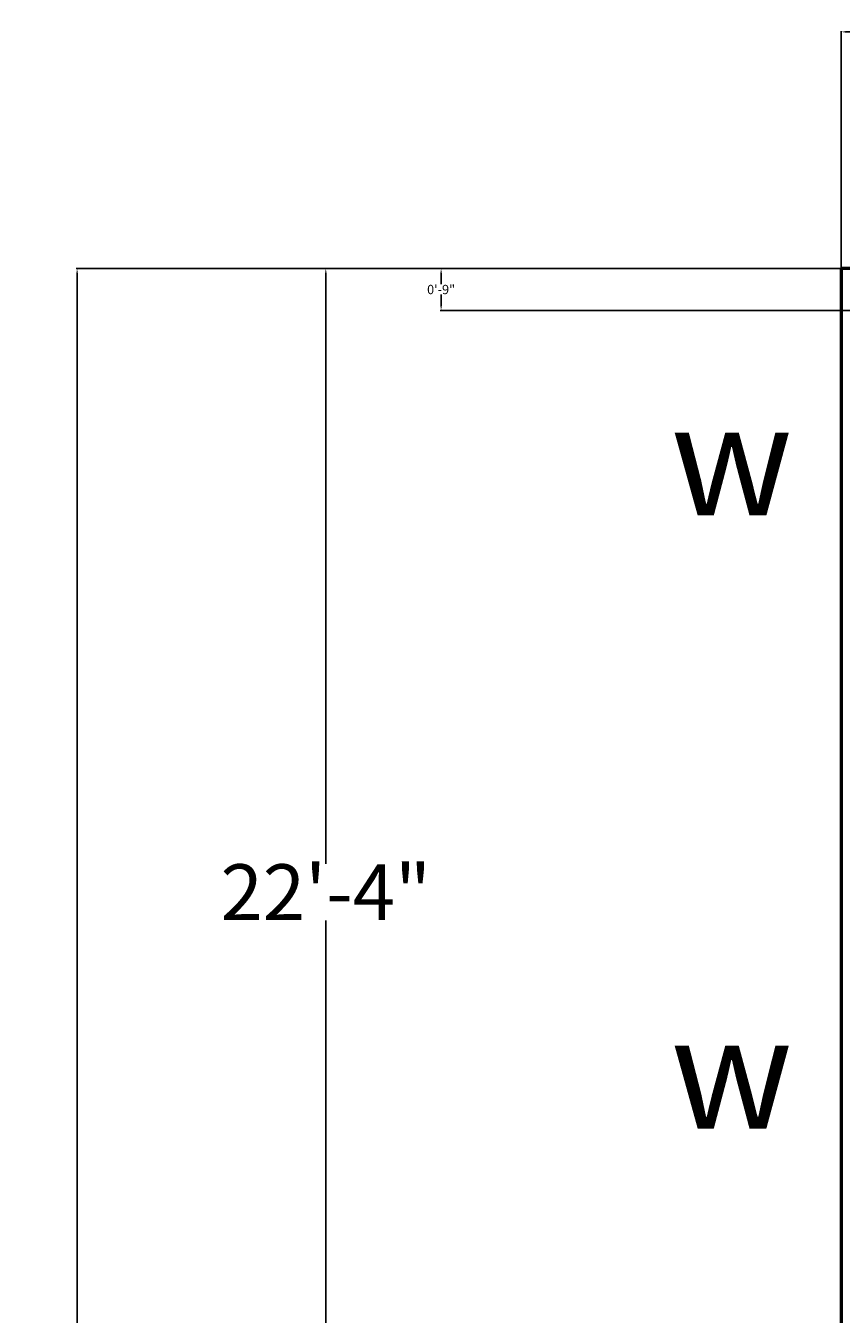
# Model space of a CAD drawing. Units: inches. Extents: x 409 to 7572, y 7 to 725.
# Tile 29 of 38: x 5502 to 5677, y 448 to 725. Entities that reach past the tile are written whole.
import ezdxf

# ---------------------------------------------------------------- set-up
doc = ezdxf.new("R2010")
doc.units = ezdxf.units.IN
doc.header["$MEASUREMENT"] = 0
for name, color, linetype, lineweight in [('A-ANNO-DIMS', 2, 'Continuous', 18), ('A-ANNO-SYMB', 3, 'Continuous', 25), ('A-WALL', 7, 'Continuous', 50)]:
    doc.layers.add(name, color=color, linetype=linetype, lineweight=lineweight)
doc.styles.get("Standard").update_dxf_attribs({"font": 'arial.ttf'})
doc.dimstyles.get("Standard").update_dxf_attribs({"dimtxt": 2, "dimasz": 1, "dimexe": 0.18, "dimexo": 0.0625, "dimgap": 0.09, "dimtad": 0, "dimtih": 1, "dimtoh": 1, "dimdec": 0, "dimzin": 0, "dimdsep": 46, "dimlunit": 3, "dimtxsty": 'Standard', "dimcen": 0.09, "dimadec": 0, "dimazin": 0, "dimtfac": 1, "dimtdec": 0, "dimtofl": 0, "dimtmove": 0, "dimatfit": 3, "dimfxl": 1, "dimtolj": 1, "dimtzin": 0, "dimarcsym": 0})

# ---------------------------------------------------------------- blocks, each defined once
blk = doc.blocks.new('*D146')
at = {"layer": 'A-ANNO-DIMS', "color": 0, "lineweight": -2, "transparency": 16777216}
for p, q in [((5676.78, 672.59), (5676.78, 723.56)), ((5677.78, 723.38), (5944.22, 723.38)), ((6217.78, 723.38), (5951.35, 723.38)), ((6218.78, 672.59), (6218.78, 723.56))]:
    blk.add_line(p, q, dxfattribs=at)
at = {"layer": 'A-ANNO-DIMS', "color": 0, "transparency": 16777216}
for points in [[(5677.78, 723.55), (5677.78, 723.22), (5676.78, 723.38)], [(6217.78, 723.55), (6217.78, 723.22), (6218.78, 723.38)]]:
    blk.add_solid(points, dxfattribs=at)
at = {"layer": 'DEFPOINTS', "color": 0, "transparency": 16777216}
for p in [(5676.78, 723.38), (5676.78, 672.53), (6218.78, 672.53)]:
    blk.add_point(p, dxfattribs=at)
at = {"layer": 'A-ANNO-DIMS', "color": 0, "transparency": 16777216, "insert": (5947.78, 723.38), "char_height": 2, "attachment_point": 5}
blk.add_mtext('\\A1;45\'-2"', dxfattribs=at)
blk = doc.blocks.new('*D132')
at = {"layer": 'A-ANNO-DIMS', "color": 0, "lineweight": -2, "transparency": 16777216}
for p, q in [((5676.72, 672.53), (5565.82, 672.53)), ((5566, 671.53), (5566, 544.65)), ((5566, 405.53), (5566, 532.42)), ((5676.72, 404.53), (5565.82, 404.53))]:
    blk.add_line(p, q, dxfattribs=at)
at = {"layer": 'A-ANNO-DIMS', "color": 0, "transparency": 16777216}
for points in [[(5565.84, 671.53), (5566.17, 671.53), (5566, 672.53)], [(5565.84, 405.53), (5566.17, 405.53), (5566, 404.53)]]:
    blk.add_solid(points, dxfattribs=at)
at = {"layer": 'DEFPOINTS', "color": 0, "transparency": 16777216}
for p in [(5676.78, 672.53), (5566, 404.53), (5676.78, 404.53)]:
    blk.add_point(p, dxfattribs=at)
at = {"layer": 'A-ANNO-DIMS', "color": 0, "transparency": 16777216, "insert": (5566, 538.53), "char_height": 2, "attachment_point": 5}
blk.add_mtext('\\A1;{\\H6x;22\'-4"}', dxfattribs=at)
blk = doc.blocks.new('*D121')
at = {"layer": 'A-ANNO-DIMS', "color": 0, "lineweight": -2, "transparency": 16777216}
for p, q in [((5676.72, 672.53), (5512.37, 672.53)), ((5512.55, 671.53), (5512.55, 420.75)), ((5512.55, 157.53), (5512.55, 408.31)), ((5676.72, 156.53), (5512.37, 156.53))]:
    blk.add_line(p, q, dxfattribs=at)
at = {"layer": 'A-ANNO-DIMS', "color": 0, "transparency": 16777216}
for points in [[(5512.38, 671.53), (5512.71, 671.53), (5512.55, 672.53)], [(5512.38, 157.53), (5512.71, 157.53), (5512.55, 156.53)]]:
    blk.add_solid(points, dxfattribs=at)
at = {"layer": 'DEFPOINTS', "color": 0, "transparency": 16777216}
for p in [(5676.78, 672.53), (5512.55, 156.53), (5676.78, 156.53)]:
    blk.add_point(p, dxfattribs=at)
at = {"layer": 'A-ANNO-DIMS', "color": 0, "transparency": 16777216, "insert": (5512.55, 414.53), "char_height": 2, "attachment_point": 5}
blk.add_mtext("\\A1;{\\H6x;43'}", dxfattribs=at)
blk = doc.blocks.new('*D192')
at = {"layer": 'A-ANNO-DIMS', "color": 0, "lineweight": -2, "transparency": 16777216}
for p, q in [((5676.72, 672.53), (5590.6, 672.53)), ((5590.78, 671.53), (5590.78, 669.14)), ((5590.78, 664.53), (5590.78, 666.92)), ((5685.72, 663.53), (5590.6, 663.53))]:
    blk.add_line(p, q, dxfattribs=at)
at = {"layer": 'A-ANNO-DIMS', "color": 0, "transparency": 16777216}
for points in [[(5590.62, 671.53), (5590.95, 671.53), (5590.78, 672.53)], [(5590.62, 664.53), (5590.95, 664.53), (5590.78, 663.53)]]:
    blk.add_solid(points, dxfattribs=at)
at = {"layer": 'DEFPOINTS', "color": 0, "transparency": 16777216}
for p in [(5676.78, 672.53), (5590.78, 663.53), (5685.78, 663.53)]:
    blk.add_point(p, dxfattribs=at)
at = {"layer": 'A-ANNO-DIMS', "color": 0, "transparency": 16777216, "insert": (5590.78, 668.03), "char_height": 2, "attachment_point": 5}
blk.add_mtext('\\A1;0\'-9"', dxfattribs=at)

msp = doc.modelspace()

# ---------------------------------------------------------------- linework, layer by layer
at = {"layer": 'A-WALL'}
for p, q in [((6218.78, 672.53), (5676.78, 672.53)), ((5676.78, 672.53), (5676.78, 404.53))]:
    msp.add_line(p, q, dxfattribs=at)

# ---------------------------------------------------------------- texts
at = {"layer": 'A-ANNO-SYMB', "char_height": 24, "attachment_point": 1}
for insert in [(5640.1, 643.49), (5640.1, 511.76)]:
    msp.add_mtext_dynamic_manual_height_columns('w', width=18.2582, gutter_width=1, heights=[0], dxfattribs=dict(at, insert=insert))

# ---------------------------------------------------------------- dimensions: what is measured, and where the dimension line sits
at = {"layer": 'A-ANNO-DIMS'}
dim = msp.add_linear_dim(base=(5676.78, 723.38), p1=(6218.78, 672.53), p2=(5676.78, 672.53), dimstyle='Standard', override={"dimclrd": 0, "dimclre": 0, "dimclrt": 0}, dxfattribs=at)
dim.commit()
dim.dimension.update_dxf_attribs({"geometry": '*D146', "text_midpoint": (5947.78, 723.38)})
for base, p2, picture, middle in [((5512.55, 156.53), (5676.78, 156.53), '*D121', (5512.55, 414.53)), ((5566, 404.53), (5676.78, 404.53), '*D132', (5566, 538.53))]:
    dim = msp.add_linear_dim(base=base, p1=(5676.78, 672.53), p2=p2, angle=90, text='{\\H6x;<>}', dimstyle='Standard', override={"dimclrd": 0, "dimclre": 0, "dimclrt": 0}, dxfattribs=at)
    dim.commit()
    dim.dimension.update_dxf_attribs({"geometry": picture, "text_midpoint": middle})
dim = msp.add_linear_dim(base=(5590.78, 663.53), p1=(5676.78, 672.53), p2=(5685.78, 663.53), angle=90, dimstyle='Standard', override={"dimdec": 1, "dimlfac": 1, "dimrnd": 0, "dimzin": 1, "dimdsep": 46, "dimlunit": 4, "dimfrac": 2}, dxfattribs=at)
dim.commit()
dim.dimension.update_dxf_attribs({"geometry": '*D192', "text_midpoint": (5590.78, 668.03)})

doc.saveas('drawing.dxf')
